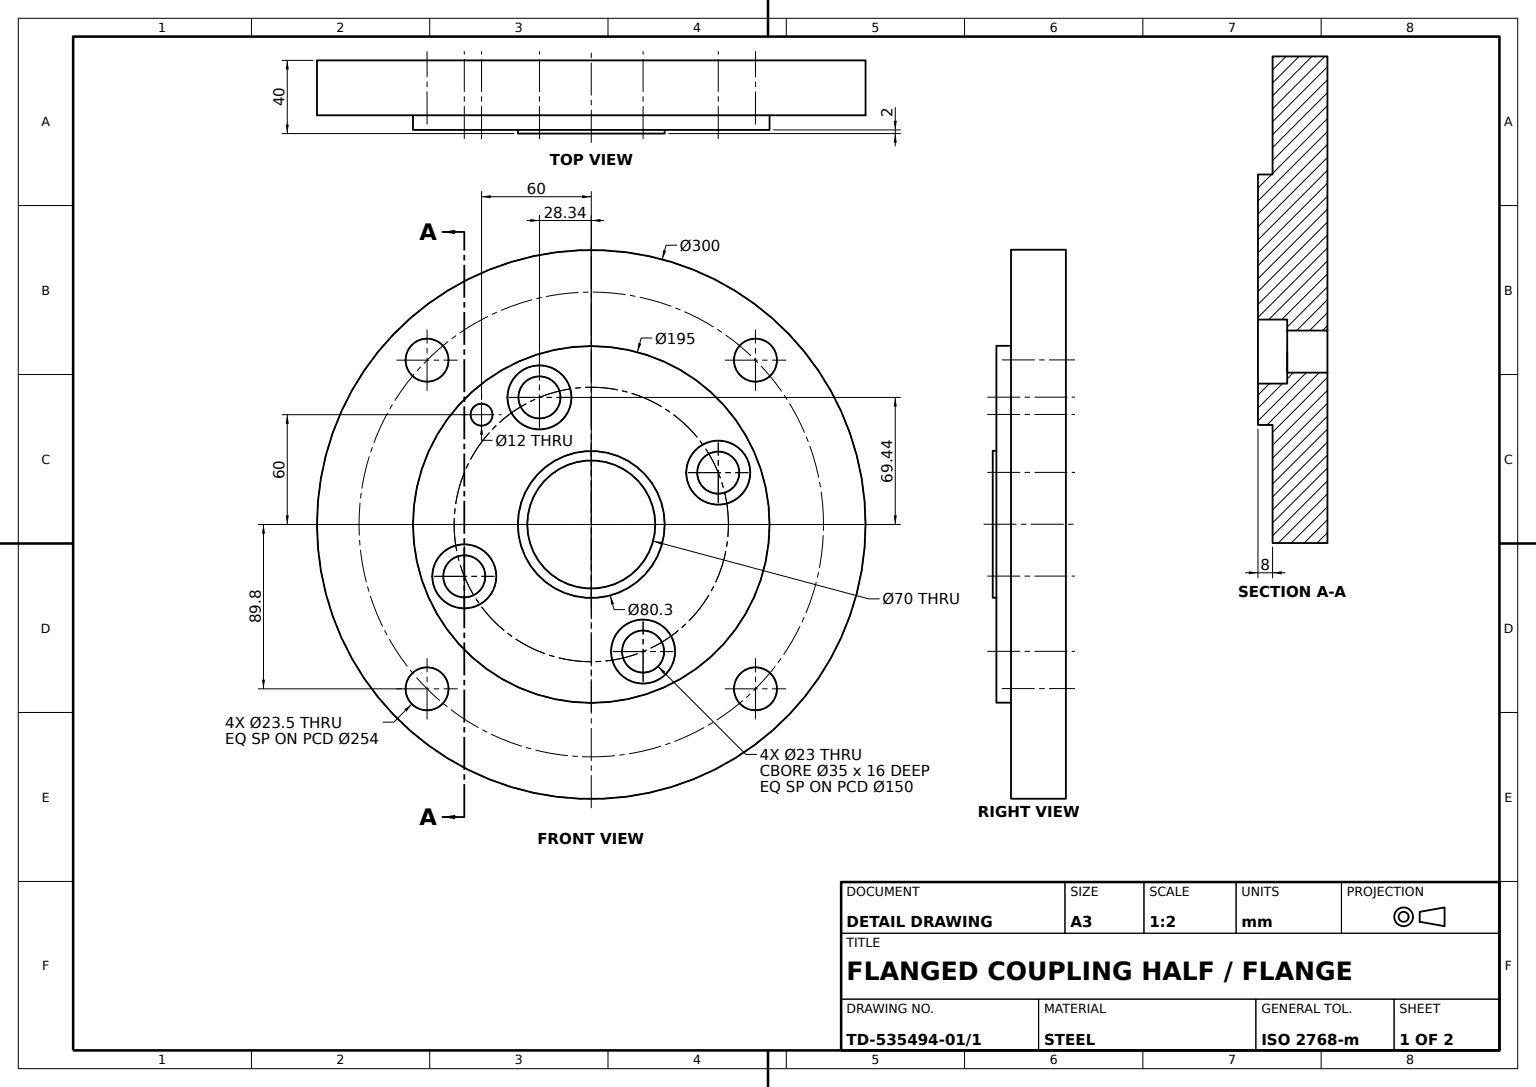
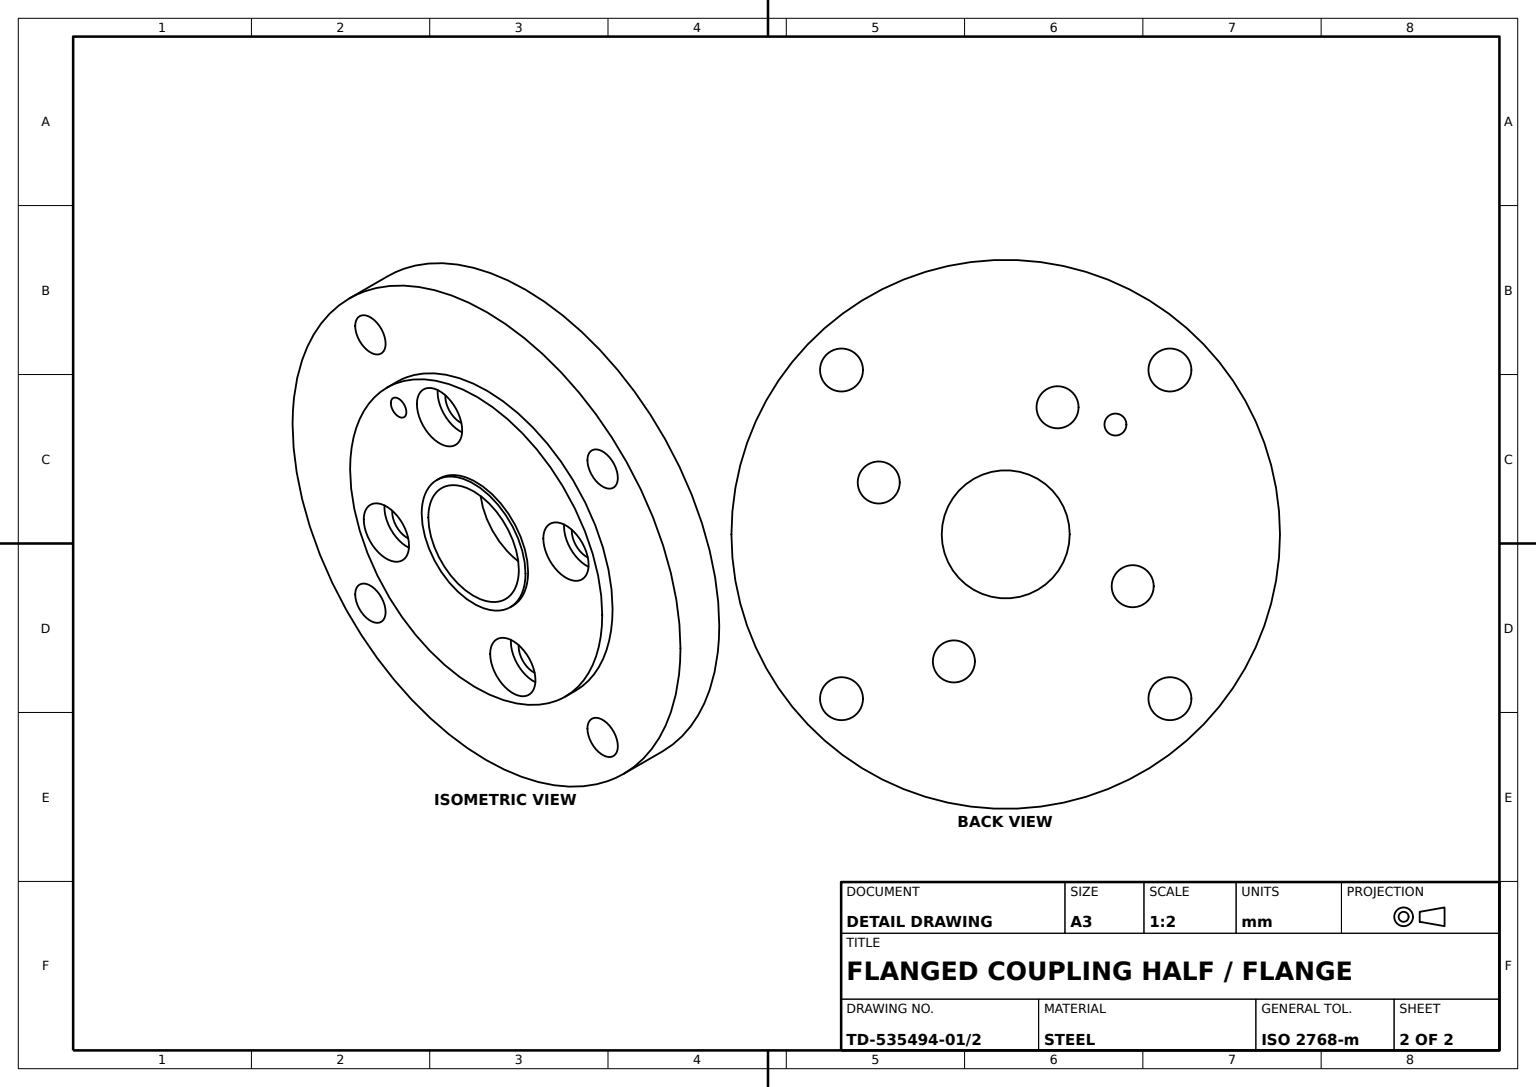
SolidWorks part; units mm, degrees
material "Plain Carbon Steel"
ref_plane "Front Plane" through (0, 0, 0) normal (0, 0, 1) x (1, 0, 0)
ref_plane "Top Plane" through (0, 0, 0) normal (0, 1, 0) x (1, 0, 0)
ref_plane "Right Plane" through (0, 0, 0) normal (1, 0, 0) x (0, 0, -1)
sketch "Flange Disc Profile" plane through (0, 0, 0) normal (0, 0, 1) x (1, 0, 0)
  circle A0 centre (0, 0) radius 150
  dimension "D1" = 300
extrude "Flange Disc Ø300" add sketch "Flange Disc Profile" along normal blind 30
sketch "Raised Face Profile" plane through (0, 0, 30) normal (0, 0, 1) x (1, 0, 0)
  circle A0 centre (0, 0) radius 97.5
  dimension "D1" = 195
extrude "Raised Face Ø195" add sketch "Raised Face Profile" along normal blind 8
sketch "Hub Spigot Profile" plane through (0, 0, 38) normal (0, 0, 1) x (1, 0, 0)
  circle A0 centre (0, 0) radius 40.15
  dimension "D1" = 80.3
extrude "Hub Spigot Ø80.3" add sketch "Hub Spigot Profile" along normal blind 2
sketch "Through Holes Profile" plane through (0, 0, 40) normal (0, 0, 1) x (1, 0, 0)
  line L0 (0, 0) -> (0, 150) construction
  line L1 (0, 0) -> (150, 0) construction
  line L2 (0, 0) -> (0, -150) construction
  line L3 (0, 0) -> (-150, 0) construction
  line L4 (0, 0) -> (-36.8395, 90.2724)
  line L5 (0, 0) -> (89.8026, 89.8026)
  line L6 (0, 0) -> (-60, 0)
  line L7 (-60, 0) -> (-60, 60)
  circle A0 centre (0, 0) radius 150 construction
  circle A1 centre (0, 0) radius 97.5
  circle A2 centre (-36.8395, 90.2724) radius 17.5
  circle A3 centre (90.2724, 36.8395) radius 17.5
  circle A4 centre (36.8395, -90.2724) radius 17.5
  circle A5 centre (-90.2724, -36.8395) radius 17.5
  circle A6 centre (0, 0) radius 127 construction
  circle A7 centre (89.8026, 89.8026) radius 11.75
  circle A8 centre (89.8026, -89.8026) radius 11.75
  circle A9 centre (-89.8026, -89.8026) radius 11.75
  circle A10 centre (-89.8026, 89.8026) radius 11.75
  circle A11 centre (-60, 60) radius 6
  dimension "D2" = 35
  dimension "D4" = 254
  dimension "D6" = 23.5
  dimension "D10" = 12
  dimension "D11" = 195
  dimension "D12" = 36.8395
  dimension "D14" = 52.9652
  dimension "D1" = 22.2
  dimension "D5" = 45
  dimension "D8" = 60
  dimension "D9" = 60
  dimension "D13" = 90.2724
  dimension "D15" = 52.9631
  dimension "D3" = 4
  dimension "D7" = 4
extrude "Through Holes PCD254" cut sketch "Through Holes Profile" against normal blind 40
sketch "Counterbore Profile" plane through (0, 0, 38) normal (0, 0, 1) x (1, 0, 0)
  line L0 (0, 0) -> (0, 97.5)
  line L1 (0, 0) -> (0, -97.5)
  line L2 (0, 0) -> (97.5, 0)
  line L3 (0, 0) -> (-97.5, 0)
  line L4 (0, 0) -> (-28.3381, 69.4403)
  circle A0 centre (0, 0) radius 97.5 construction
  circle A2 centre (0, 0) radius 75
  circle A3 centre (-28.3381, 69.4403) radius 17.5
  circle A4 centre (69.4403, 28.3381) radius 17.5
  circle A5 centre (28.3381, -69.4403) radius 17.5
  circle A6 centre (-69.4403, -28.3381) radius 17.5
  dimension "D2" = 150
  dimension "D3" = 35
  dimension "D1" = 22.2
  dimension "D5" = 28.3381
  dimension "D6" = 69.4403
  dimension "D4" = 4
extrude "Counterbores 4xØ35" cut sketch "Counterbore Profile" against normal blind 16 contours A2 A6 | A2 A6 | A2 A3 | A2 A3 L4 | L4 A3 A2 | A2 A4 | A2 A4 | A2 A5 | A2 A5
sketch "Counterbored Holes Profile" plane through (0, 0, 22) normal (0, 0, 1) x (1, 0, 0)
  circle A0 centre (-28.3381, 69.4403) radius 11.5
  circle A1 centre (69.4403, 28.3381) radius 11.5
  circle A2 centre (28.3381, -69.4403) radius 11.5
  circle A3 centre (-69.4403, -28.3381) radius 11.5
  dimension "D1" = 23
  dimension "D3" = 75
  dimension "D4" = 28.3381
  dimension "D2" = 4
extrude "Counterbored Holes 4xØ23" cut sketch "Counterbored Holes Profile" against normal blind 30
sketch "Central Bore Profile" plane through (0, 0, 40) normal (0, 0, 1) x (1, 0, 0)
  circle A0 centre (0, 0) radius 35
  dimension "D1" = 70
extrude "Central Bore Ø70" cut sketch "Central Bore Profile" against normal blind 50
